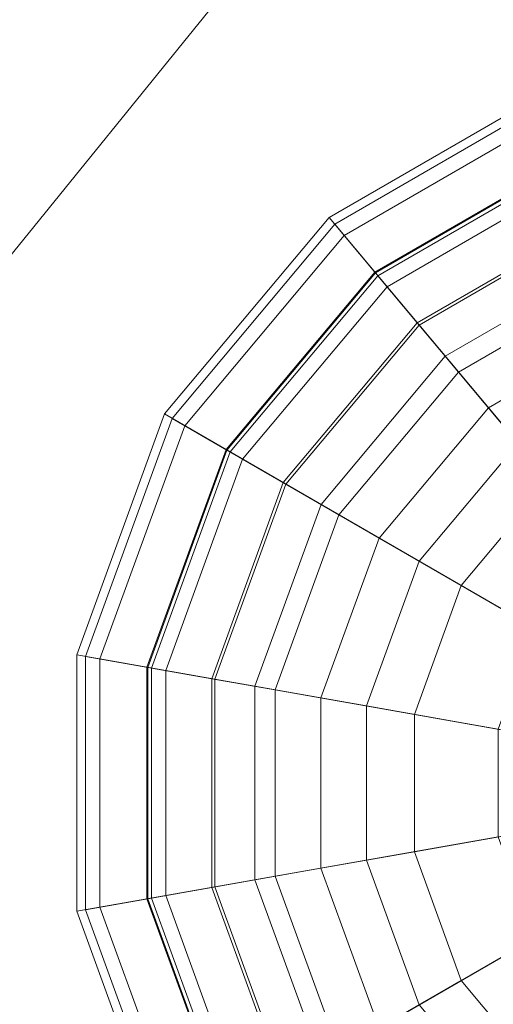
# Model space of a CAD drawing. Units: inches. Extents: x 375 to 1122, y 27 to 1069.
# Tile 91 of 155: x 728.243 to 729.113, y 860.072 to 861.878. Entities that reach past the tile are written whole.
import ezdxf

# ---------------------------------------------------------------- set-up
doc = ezdxf.new("R2010")
doc.units = ezdxf.units.IN
doc.layers.add('A-ANNO-DIMS', color=2, linetype='Continuous', lineweight=18)
doc.layers.add('Furniture', color=30, linetype='Continuous', lineweight=18)
doc.styles.get("Standard").update_dxf_attribs({"font": 'arial.ttf'})
doc.dimstyles.new('ISO-25', dxfattribs={"dimtxt": 12, "dimasz": 2.5, "dimexe": 1.5, "dimexo": 1.5, "dimtad": 1, "dimdec": 1, "dimlunit": 3, "dimtxsty": 'Standard', "dimblk": 'ARCHTICK', "dimcen": 2.5, "dimadec": 0, "dimazin": 0, "dimtfac": 1, "dimtdec": 1, "dimtmove": 0, "dimatfit": 3, "dimfxl": 1.5, "dimfxlon": 1, "dimarcsym": 0})

# ---------------------------------------------------------------- blocks, each defined once
blk = doc.blocks.new('A$C403C54AD')
blk.add_line((1.789224, 1.189932, 0.036628), (1.95298, 1.056939, 0.036628))
for points in [[(1.914522, 1.106811, -0.060915), (1.946342, 1.118392, -0.057836), (1.946342, 1.118392, -0.057836), (1.920403, 1.096626, -0.060915)], [(1.920403, 1.096626, -0.060915), (1.946342, 1.118392, -0.057836), (1.946342, 1.118392, -0.057836), (1.929411, 1.089067, -0.060915)], [(1.929411, 1.089067, -0.060915), (1.946342, 1.118392, -0.057836), (1.946342, 1.118392, -0.057836), (1.940462, 1.085044, -0.060915)], [(1.940462, 1.085044, -0.060915), (1.946342, 1.118392, -0.057836), (1.946342, 1.118392, -0.057836), (1.952223, 1.085044, -0.060915)], [(1.972282, 1.096626, -0.060915), (1.946342, 1.118392, -0.057836), (1.946342, 1.118392, -0.057836), (1.978163, 1.106811, -0.060915)], [(1.963274, 1.089067, -0.060915), (1.946342, 1.118392, -0.057836), (1.946342, 1.118392, -0.057836), (1.972282, 1.096626, -0.060915)], [(1.952223, 1.085044, -0.060915), (1.946342, 1.118392, -0.057836), (1.946342, 1.118392, -0.057836), (1.963274, 1.089067, -0.060915)], [(1.932985, 1.113531, -0.054409), (1.917591, 1.107928, -0.057684), (1.922904, 1.098725, -0.057684), (1.935454, 1.109255, -0.054409)], [(1.939522, 1.112669, 0.027913), (1.932456, 1.10674, 0.03455), (1.937279, 1.102693, 0.03455), (1.94189, 1.110681, 0.027913)], [(1.950795, 1.110681, 0.027913), (1.955406, 1.102693, 0.03455), (1.960229, 1.10674, 0.03455), (1.953163, 1.112669, 0.027913)], [(1.929308, 1.112192, 0.03455), (1.923214, 1.109974, 0.043942), (1.927488, 1.102571, 0.043942), (1.932456, 1.10674, 0.03455)], [(1.930748, 1.105307, 0.032362), (1.938591, 1.111888, 0.024995), (1.941283, 1.109629, 0.024995), (1.936164, 1.100762, 0.032362)], [(1.956521, 1.100762, 0.032362), (1.951402, 1.109629, 0.024995), (1.954094, 1.111888, 0.024995), (1.961937, 1.105307, 0.032362)], [(1.920572, 1.109013, 0.042594), (1.927213, 1.111429, 0.032362), (1.930748, 1.105307, 0.032362), (1.925335, 1.100764, 0.042594)], [(1.920436, 1.108963, 0.101264), (1.925217, 1.110703, 0.111475), (1.929121, 1.103941, 0.111475), (1.925223, 1.100671, 0.101264)], [(1.925217, 1.110703, 0.111475), (1.922324, 1.10965, 0.111475), (1.926763, 1.101963, 0.111475), (1.929121, 1.103941, 0.111475)], [(1.94189, 1.110681, 0.027913), (1.937279, 1.102693, 0.03455), (1.943195, 1.10054, 0.03455), (1.944796, 1.109623, 0.027913)], [(1.947889, 1.109623, 0.027913), (1.94949, 1.10054, 0.03455), (1.955406, 1.102693, 0.03455), (1.950795, 1.110681, 0.027913)], [(1.923214, 1.109974, 0.043942), (1.918414, 1.108227, 0.061088), (1.923575, 1.099288, 0.061088), (1.927488, 1.102571, 0.043942)], [(1.922324, 1.10965, 0.111475), (1.917629, 1.107941, 0.102069), (1.922935, 1.098751, 0.102069), (1.926763, 1.101963, 0.111475)], [(1.936164, 1.100762, 0.032362), (1.941283, 1.109629, 0.024995), (1.944585, 1.108427, 0.024995), (1.942807, 1.098344, 0.032362)], [(1.944796, 1.109623, 0.027913), (1.943195, 1.10054, 0.03455), (1.94949, 1.10054, 0.03455), (1.947889, 1.109623, 0.027913)], [(1.949878, 1.098344, 0.032362), (1.9481, 1.108427, 0.024995), (1.951402, 1.109629, 0.024995), (1.956521, 1.100762, 0.032362)], [(1.915531, 1.107178, 0.060603), (1.920572, 1.109013, 0.042594), (1.925335, 1.100764, 0.042594), (1.921225, 1.097316, 0.060603)], [(1.917796, 1.108002, 0.088628), (1.920436, 1.108963, 0.101264), (1.925223, 1.100671, 0.101264), (1.923071, 1.098865, 0.088628)], [(1.935454, 1.109255, -0.054409), (1.922904, 1.098725, -0.057684), (1.931044, 1.091895, -0.057684), (1.939235, 1.106082, -0.054409)], [(1.95345, 1.106082, -0.054409), (1.961641, 1.091895, -0.057684), (1.969781, 1.098725, -0.057684), (1.957231, 1.109255, -0.054409)], [(1.918414, 1.108227, 0.061088), (1.917796, 1.108002, 0.088628), (1.923071, 1.098865, 0.088628), (1.923575, 1.099288, 0.061088)], [(1.942807, 1.098344, 0.032362), (1.944585, 1.108427, 0.024995), (1.9481, 1.108427, 0.024995), (1.949878, 1.098344, 0.032362)], [(1.917591, 1.107928, -0.057684), (1.914522, 1.106811, -0.060915), (1.920403, 1.096626, -0.060915), (1.922904, 1.098725, -0.057684)], [(1.917629, 1.107941, 0.102069), (1.914897, 1.106947, 0.088845), (1.920708, 1.096882, 0.088845), (1.922935, 1.098751, 0.102069)], [(1.914897, 1.106947, 0.088845), (1.915531, 1.107178, 0.060603), (1.921225, 1.097316, 0.060603), (1.920708, 1.096882, 0.088845)], [(1.932456, 1.10674, 0.03455), (1.927488, 1.102571, 0.043942), (1.934036, 1.097077, 0.043942), (1.937279, 1.102693, 0.03455)], [(1.955406, 1.102693, 0.03455), (1.958649, 1.097077, 0.043942), (1.965197, 1.102571, 0.043942), (1.960229, 1.10674, 0.03455)], [(1.939235, 1.106082, -0.054409), (1.931044, 1.091895, -0.057684), (1.941029, 1.088261, -0.057684), (1.943874, 1.104394, -0.054409)], [(1.948811, 1.104394, -0.054409), (1.951655, 1.088261, -0.057684), (1.961641, 1.091895, -0.057684), (1.95345, 1.106082, -0.054409)], [(1.925335, 1.100764, 0.042594), (1.930748, 1.105307, 0.032362), (1.936164, 1.100762, 0.032362), (1.932631, 1.094642, 0.042594)], [(1.943874, 1.104394, -0.054409), (1.941029, 1.088261, -0.057684), (1.951655, 1.088261, -0.057684), (1.948811, 1.104394, -0.054409)], [(1.925223, 1.100671, 0.101264), (1.929121, 1.103941, 0.111475), (1.935102, 1.098923, 0.111475), (1.932558, 1.094517, 0.101264)], [(1.929121, 1.103941, 0.111475), (1.926763, 1.101963, 0.111475), (1.933563, 1.096257, 0.111475), (1.935102, 1.098923, 0.111475)], [(1.937279, 1.102693, 0.03455), (1.934036, 1.097077, 0.043942), (1.942068, 1.094153, 0.043942), (1.943195, 1.10054, 0.03455)], [(1.94949, 1.10054, 0.03455), (1.950616, 1.094153, 0.043942), (1.958649, 1.097077, 0.043942), (1.955406, 1.102693, 0.03455)], [(1.927488, 1.102571, 0.043942), (1.923575, 1.099288, 0.061088), (1.931482, 1.092653, 0.061088), (1.934036, 1.097077, 0.043942)], [(1.926763, 1.101963, 0.111475), (1.922935, 1.098751, 0.102069), (1.931064, 1.09193, 0.102069), (1.933563, 1.096257, 0.111475)], [(1.921225, 1.097316, 0.060603), (1.925335, 1.100764, 0.042594), (1.932631, 1.094642, 0.042594), (1.929948, 1.089997, 0.060603)], [(1.923071, 1.098865, 0.088628), (1.925223, 1.100671, 0.101264), (1.932558, 1.094517, 0.101264), (1.931153, 1.092083, 0.088628)], [(1.932631, 1.094642, 0.042594), (1.936164, 1.100762, 0.032362), (1.942807, 1.098344, 0.032362), (1.94158, 1.091385, 0.042594)], [(1.943195, 1.10054, 0.03455), (1.942068, 1.094153, 0.043942), (1.950616, 1.094153, 0.043942), (1.94949, 1.10054, 0.03455)], [(1.951105, 1.091385, 0.042594), (1.949878, 1.098344, 0.032362), (1.956521, 1.100762, 0.032362), (1.960054, 1.094642, 0.042594)], [(1.923575, 1.099288, 0.061088), (1.923071, 1.098865, 0.088628), (1.931153, 1.092083, 0.088628), (1.931482, 1.092653, 0.061088)], [(1.922904, 1.098725, -0.057684), (1.920403, 1.096626, -0.060915), (1.929411, 1.089067, -0.060915), (1.931044, 1.091895, -0.057684)], [(1.922935, 1.098751, 0.102069), (1.920708, 1.096882, 0.088845), (1.929611, 1.089412, 0.088845), (1.931064, 1.09193, 0.102069)], [(1.932558, 1.094517, 0.101264), (1.935102, 1.098923, 0.111475), (1.942439, 1.096252, 0.111475), (1.941555, 1.091242, 0.101264)], [(1.935102, 1.098923, 0.111475), (1.933563, 1.096257, 0.111475), (1.941904, 1.093221, 0.111475), (1.942439, 1.096252, 0.111475)], [(1.950246, 1.096252, 0.111475), (1.950781, 1.093221, 0.111475), (1.959122, 1.096257, 0.111475), (1.957583, 1.098923, 0.111475)], [(1.95113, 1.091242, 0.101264), (1.950246, 1.096252, 0.111475), (1.957583, 1.098923, 0.111475), (1.960127, 1.094517, 0.101264)], [(1.94158, 1.091385, 0.042594), (1.942807, 1.098344, 0.032362), (1.949878, 1.098344, 0.032362), (1.951105, 1.091385, 0.042594)], [(1.920708, 1.096882, 0.088845), (1.921225, 1.097316, 0.060603), (1.929948, 1.089997, 0.060603), (1.929611, 1.089412, 0.088845)], [(1.934036, 1.097077, 0.043942), (1.931482, 1.092653, 0.061088), (1.941182, 1.089123, 0.061088), (1.942068, 1.094153, 0.043942)], [(1.950616, 1.094153, 0.043942), (1.951503, 1.089123, 0.061088), (1.961203, 1.092653, 0.061088), (1.958649, 1.097077, 0.043942)], [(1.933563, 1.096257, 0.111475), (1.931064, 1.09193, 0.102069), (1.941036, 1.0883, 0.102069), (1.941904, 1.093221, 0.111475)], [(1.941555, 1.091242, 0.101264), (1.942439, 1.096252, 0.111475), (1.950246, 1.096252, 0.111475), (1.95113, 1.091242, 0.101264)], [(1.942439, 1.096252, 0.111475), (1.941904, 1.093221, 0.111475), (1.950781, 1.093221, 0.111475), (1.950246, 1.096252, 0.111475)], [(1.950781, 1.093221, 0.111475), (1.951648, 1.0883, 0.102069), (1.96162, 1.09193, 0.102069), (1.959122, 1.096257, 0.111475)], [(1.929948, 1.089997, 0.060603), (1.932631, 1.094642, 0.042594), (1.94158, 1.091385, 0.042594), (1.940649, 1.086102, 0.060603)], [(1.931153, 1.092083, 0.088628), (1.932558, 1.094517, 0.101264), (1.941555, 1.091242, 0.101264), (1.941067, 1.088475, 0.088628)], [(1.952036, 1.086102, 0.060603), (1.951105, 1.091385, 0.042594), (1.960054, 1.094642, 0.042594), (1.962737, 1.089997, 0.060603)], [(1.951618, 1.088475, 0.088628), (1.95113, 1.091242, 0.101264), (1.960127, 1.094517, 0.101264), (1.961532, 1.092083, 0.088628)], [(1.942068, 1.094153, 0.043942), (1.941182, 1.089123, 0.061088), (1.951503, 1.089123, 0.061088), (1.950616, 1.094153, 0.043942)], [(1.941904, 1.093221, 0.111475), (1.941036, 1.0883, 0.102069), (1.951648, 1.0883, 0.102069), (1.950781, 1.093221, 0.111475)], [(1.931482, 1.092653, 0.061088), (1.931153, 1.092083, 0.088628), (1.941067, 1.088475, 0.088628), (1.941182, 1.089123, 0.061088)], [(1.951503, 1.089123, 0.061088), (1.951618, 1.088475, 0.088628), (1.961532, 1.092083, 0.088628), (1.961203, 1.092653, 0.061088)], [(1.931044, 1.091895, -0.057684), (1.929411, 1.089067, -0.060915), (1.940462, 1.085044, -0.060915), (1.941029, 1.088261, -0.057684)], [(1.931064, 1.09193, 0.102069), (1.929611, 1.089412, 0.088845), (1.940532, 1.085437, 0.088845), (1.941036, 1.0883, 0.102069)], [(1.951648, 1.0883, 0.102069), (1.952153, 1.085437, 0.088845), (1.963074, 1.089412, 0.088845), (1.96162, 1.09193, 0.102069)], [(1.951655, 1.088261, -0.057684), (1.952223, 1.085044, -0.060915), (1.963274, 1.089067, -0.060915), (1.961641, 1.091895, -0.057684)], [(1.940649, 1.086102, 0.060603), (1.94158, 1.091385, 0.042594), (1.951105, 1.091385, 0.042594), (1.952036, 1.086102, 0.060603)], [(1.941067, 1.088475, 0.088628), (1.941555, 1.091242, 0.101264), (1.95113, 1.091242, 0.101264), (1.951618, 1.088475, 0.088628)], [(1.929611, 1.089412, 0.088845), (1.929948, 1.089997, 0.060603), (1.940649, 1.086102, 0.060603), (1.940532, 1.085437, 0.088845)], [(1.952153, 1.085437, 0.088845), (1.952036, 1.086102, 0.060603), (1.962737, 1.089997, 0.060603), (1.963074, 1.089412, 0.088845)], [(1.941182, 1.089123, 0.061088), (1.941067, 1.088475, 0.088628), (1.951618, 1.088475, 0.088628), (1.951503, 1.089123, 0.061088)], [(1.941029, 1.088261, -0.057684), (1.940462, 1.085044, -0.060915), (1.952223, 1.085044, -0.060915), (1.951655, 1.088261, -0.057684)], [(1.941036, 1.0883, 0.102069), (1.940532, 1.085437, 0.088845), (1.952153, 1.085437, 0.088845), (1.951648, 1.0883, 0.102069)], [(1.940532, 1.085437, 0.088845), (1.940649, 1.086102, 0.060603), (1.952036, 1.086102, 0.060603), (1.952153, 1.085437, 0.088845)]]:
    blk.add_3dface(points)
blk = doc.blocks.new('_ArchTick')
at = {"color": 0, "linetype": 'ByBlock', "const_width": 0.15}
blk.add_lwpolyline([(-0.5, -0.5), (0.5, 0.5)], dxfattribs=at)
blk = doc.blocks.new('*D85')
at = {"layer": 'A-ANNO-DIMS', "color": 0, "lineweight": -2, "transparency": 16777216}
for p, q in [((401.5073, 868.5277), (398.5073, 868.5277)), ((400.0073, 814.5277), (400.0073, 868.5277)), ((401.5073, 814.5277), (398.5073, 814.5277))]:
    blk.add_line(p, q, dxfattribs=at)
at = {"layer": 'Defpoints', "color": 0, "transparency": 16777216}
for p in [(400.0073, 868.5277), (845.0073, 868.5277), (845.0073, 814.5277)]:
    blk.add_point(p, dxfattribs=at)
at = {"layer": 'A-ANNO-DIMS', "color": 0, "lineweight": -2, "transparency": 16777216, "xscale": 2.5, "yscale": 2.5, "zscale": 2.5}
for p, rotation in [((400.0073, 868.5277), 90), ((400.0073, 814.5277), 270)]:
    blk.add_blockref('_ArchTick', p, dxfattribs=dict(at, rotation=rotation))
at = {"layer": 'A-ANNO-DIMS', "color": 0, "transparency": 16777216, "insert": (393.2555, 841.5277), "char_height": 12, "attachment_point": 5, "rotation": 90}
blk.add_mtext('4\'-6"', dxfattribs=at)
blk = doc.blocks.new('*D91')
at = {"layer": 'A-ANNO-DIMS', "color": 0, "lineweight": -2, "transparency": 16777216}
for p, q in [((728.0073, 1052.5277), (728.0073, 1055.5277)), ((788.0073, 1052.5277), (788.0073, 1055.5277)), ((728.0073, 1054.0277), (788.0073, 1054.0277))]:
    blk.add_line(p, q, dxfattribs=at)
at = {"layer": 'Defpoints', "color": 0, "transparency": 16777216}
for p in [(788.0073, 1054.0277), (728.0073, 774.0277), (788.0073, 774.0277)]:
    blk.add_point(p, dxfattribs=at)
at = {"layer": 'A-ANNO-DIMS', "color": 0, "lineweight": -2, "transparency": 16777216, "xscale": 2.5, "yscale": 2.5, "zscale": 2.5, "rotation": 180}
blk.add_blockref('_ArchTick', (728.0073, 1054.0277), dxfattribs=at)
at = {"layer": 'A-ANNO-DIMS', "color": 0, "lineweight": -2, "transparency": 16777216, "xscale": 2.5, "yscale": 2.5, "zscale": 2.5}
blk.add_blockref('_ArchTick', (788.0073, 1054.0277), dxfattribs=at)
at = {"layer": 'A-ANNO-DIMS', "color": 0, "transparency": 16777216, "insert": (758.0073, 1060.7796), "char_height": 12, "attachment_point": 5}
blk.add_mtext('5\'-0"', dxfattribs=at)

msp = doc.modelspace()

# ---------------------------------------------------------------- block references
at = {"layer": 'Furniture', "xscale": 39.9918517141215, "yscale": 39.9918517141215, "zscale": 39.9918517141215, "rotation": 270}
msp.add_blockref('A$C403C54AD', (684.9549, 938.3156, 0.024), dxfattribs=at)

# ---------------------------------------------------------------- dimensions: what is measured, and where the dimension line sits
at = {"layer": 'A-ANNO-DIMS'}
dim = msp.add_linear_dim(base=(788.0073, 1054.0277), p1=(728.0073, 774.0277), p2=(788.0073, 774.0277), dimstyle='ISO-25', override={"dimdec": 1, "dimlfac": 1, "dimrnd": 0, "dimzin": 1, "dimdsep": 46, "dimlunit": 4, "dimfrac": 2}, dxfattribs=at)
dim.commit()
dim.dimension.update_dxf_attribs({"geometry": '*D91', "text_midpoint": (758.0073, 1060.7796)})
dim = msp.add_linear_dim(base=(400.0073, 868.5277), p1=(845.0073, 814.5277), p2=(845.0073, 868.5277), angle=90, dimstyle='ISO-25', override={"dimdec": 1, "dimlfac": 1, "dimrnd": 0, "dimzin": 1, "dimdsep": 46, "dimlunit": 4, "dimfrac": 2}, dxfattribs=at)
dim.commit()
dim.dimension.update_dxf_attribs({"geometry": '*D85', "text_midpoint": (393.2555, 841.5277)})

doc.saveas('drawing.dxf')
